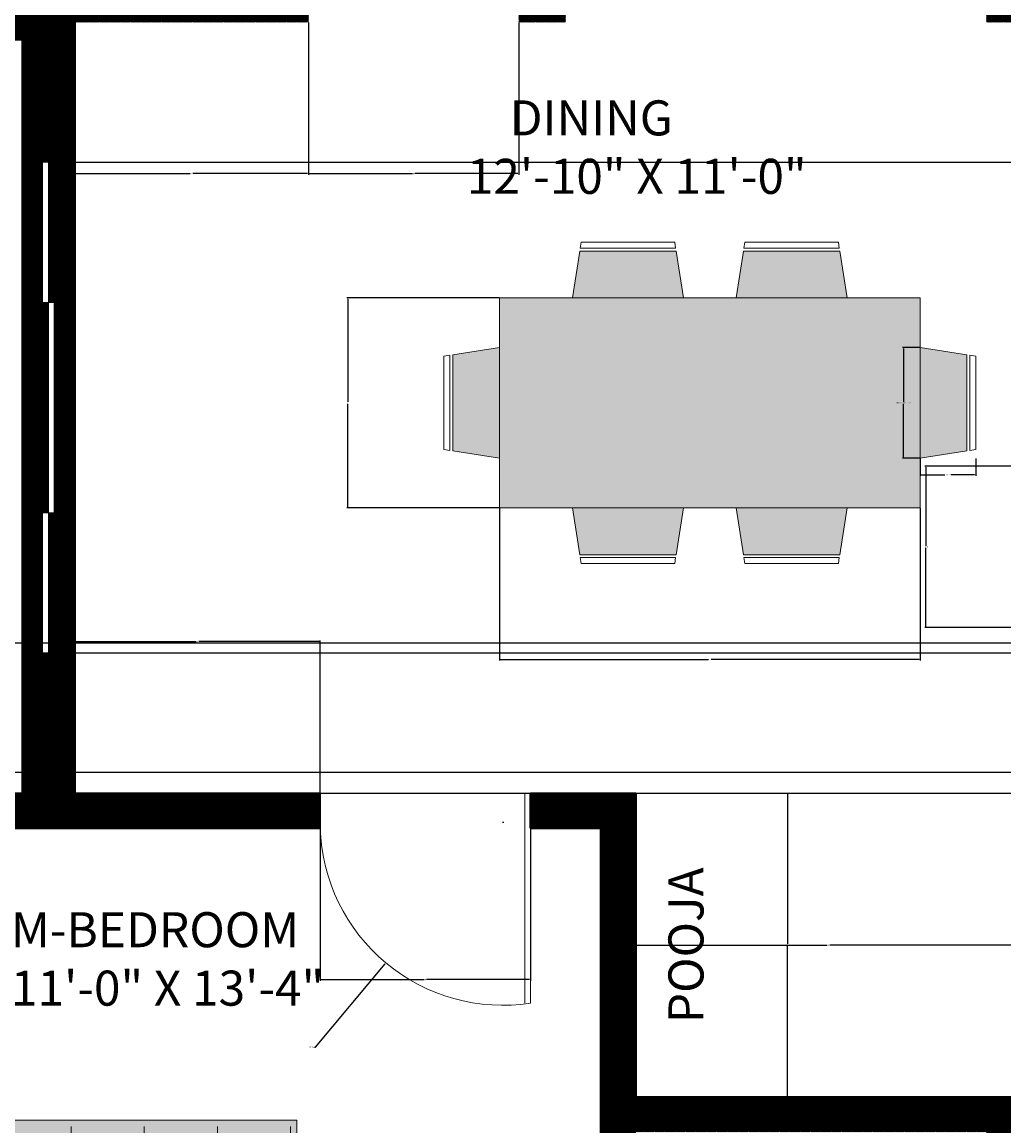
# Model space of a CAD drawing. Units: inches. Extents: x 557 to 1007, y 390 to 953.
# Tile 4 of 10: x 674 to 842, y 558 to 747. Entities that reach past the tile are written whole.
import ezdxf

# ---------------------------------------------------------------- set-up
doc = ezdxf.new("R2010")
doc.units = ezdxf.units.IN
doc.header["$LTSCALE"] = 5
doc.header["$MEASUREMENT"] = 0
for name, color, linetype, lineweight in [('A-ANNO-DIMS', 2, 'Continuous', 18), ('A-AREA-IDEN', 7, 'Continuous', 18), ('A-DOOR', 3, 'Continuous', 18), ('A-FURN', 8, 'Continuous', 18), ('A-FURN-PATT', 9, 'Continuous', 9), ('A-WALL', 7, 'Continuous', 35)]:
    doc.layers.add(name, color=color, linetype=linetype, lineweight=lineweight)
doc.layers.add('A-GLAZ-PATT', color=141, linetype='Continuous', lineweight=9, true_color=0xadddf7)
doc.layers.add('A-WALL-PATT', color=251, linetype='Continuous', lineweight=9, true_color=0x636466)
doc.styles.get("Standard").update_dxf_attribs({"font": 'arial.ttf'})
doc.dimstyles.get("Standard").update_dxf_attribs({"dimtxt": 0.18, "dimasz": 0.18, "dimexe": 0.18, "dimexo": 0.0625, "dimgap": 0.09, "dimtad": 0, "dimtih": 1, "dimtoh": 1, "dimdec": 4, "dimzin": 0, "dimdsep": 46, "dimtxsty": 'Standard', "dimcen": 0.09, "dimadec": 0, "dimazin": 0, "dimtfac": 1, "dimtdec": 4, "dimtofl": 0, "dimtmove": 0, "dimatfit": 3, "dimfxl": 1, "dimtolj": 1, "dimtzin": 0, "dimarcsym": 0})

# ---------------------------------------------------------------- blocks, each defined once
blk = doc.blocks.new('BED-QUEEN-60x80-PLAN')
for p, q in [((0, 0), (0, 60)), ((0, 60), (80, 60)), ((29.6, 60), (14.4, 44.8)), ((29.6, 44.8), (29.6, 60)), ((80, 60), (80, 0)), ((1.2, 52), (16.4, 52)), ((1.2, 31.2), (1.2, 52)), ((16.4, 52), (16.4, 46.8)), ((14.4, 0), (14.4, 44.8)), ((14.4, 44.8), (29.6, 44.8)), ((16.8, 44.8), (16.8, 0)), ((14.4, 31.2), (1.2, 31.2)), ((1.2, 28.8), (14.4, 28.8)), ((1.2, 8), (1.2, 28.8)), ((14.4, 8), (1.2, 8)), ((80, 0), (0, 0))]:
    blk.add_line(p, q)
blk = doc.blocks.new('CHAIR-DINING-PLAN')
for p, q in [((1.48, 9.5), (1.33, 8.5)), ((1.48, 9.5), (17.48, 9.5)), ((17.64, 8.5), (17.48, 9.5)), ((1.25, 8), (0, 0)), ((1.25, 8), (17.72, 8)), ((17.64, 8.5), (1.33, 8.5)), ((18.97, 0), (17.72, 8))]:
    blk.add_line(p, q)
blk = doc.blocks.new('*D25')
at = {"layer": 'A-ANNO-DIMS', "color": 0, "lineweight": -2, "ltscale": 5, "transparency": 16777216}
for p, q in [((828.02, 691.19), (825.05, 691.19)), ((825.23, 691.01), (825.23, 681.89)), ((825.23, 672.41), (825.23, 681.53)), ((828.02, 672.23), (825.05, 672.23))]:
    blk.add_line(p, q, dxfattribs=at)
at = {"layer": 'A-ANNO-DIMS', "color": 0, "ltscale": 5, "transparency": 16777216}
for points in [[(825.2, 691.01), (825.26, 691.01), (825.23, 691.19)], [(825.2, 672.41), (825.26, 672.41), (825.23, 672.23)]]:
    blk.add_solid(points, dxfattribs=at)
at = {"layer": 'Defpoints', "color": 0, "ltscale": 5, "transparency": 16777216}
for p in [(828.08, 691.19), (825.23, 672.23), (828.08, 672.23)]:
    blk.add_point(p, dxfattribs=at)
at = {"layer": 'A-ANNO-DIMS', "color": 0, "ltscale": 5, "transparency": 16777216, "insert": (825.23, 681.71), "char_height": 0.18, "attachment_point": 5}
blk.add_mtext('\\A1;DINING CHAIR 19 TYP.', dxfattribs=at)
blk = doc.blocks.new('*D26')
at = {"layer": 'A-ANNO-DIMS', "color": 0, "lineweight": -2, "ltscale": 5, "transparency": 16777216}
for p, q in [((828.08, 672.16), (828.08, 669.2)), ((837.58, 672.16), (837.58, 669.2)), ((828.26, 669.38), (832.31, 669.38)), ((837.4, 669.38), (833.35, 669.38))]:
    blk.add_line(p, q, dxfattribs=at)
at = {"layer": 'A-ANNO-DIMS', "color": 0, "ltscale": 5, "transparency": 16777216}
for points in [[(828.26, 669.41), (828.26, 669.35), (828.08, 669.38)], [(837.4, 669.41), (837.4, 669.35), (837.58, 669.38)]]:
    blk.add_solid(points, dxfattribs=at)
at = {"layer": 'Defpoints', "color": 0, "ltscale": 5, "transparency": 16777216}
for p in [(828.08, 672.23), (837.58, 672.23), (837.58, 669.38)]:
    blk.add_point(p, dxfattribs=at)
at = {"layer": 'A-ANNO-DIMS', "color": 0, "ltscale": 5, "transparency": 16777216, "insert": (832.83, 669.38), "char_height": 0.18, "attachment_point": 5}
blk.add_mtext('\\A1;10 TYP.', dxfattribs=at)
blk = doc.blocks.new('*D45')
at = {"layer": 'A-ANNO-DIMS', "color": 0, "lineweight": -2, "ltscale": 5, "transparency": 16777216}
for p, q in [((582.82, 605.84), (582.82, 389.77)), ((980.41, 439.84), (980.41, 389.77)), ((583, 389.95), (781.22, 389.95)), ((980.23, 389.95), (782.01, 389.95))]:
    blk.add_line(p, q, dxfattribs=at)
at = {"layer": 'A-ANNO-DIMS', "color": 0, "ltscale": 5, "transparency": 16777216}
for points in [[(583, 389.98), (583, 389.92), (582.82, 389.95)], [(980.23, 389.98), (980.23, 389.92), (980.41, 389.95)]]:
    blk.add_solid(points, dxfattribs=at)
at = {"layer": 'Defpoints', "color": 0, "ltscale": 5, "transparency": 16777216}
for p in [(582.82, 605.9), (980.41, 439.9), (980.41, 389.95)]:
    blk.add_point(p, dxfattribs=at)
at = {"layer": 'A-ANNO-DIMS', "color": 0, "ltscale": 5, "transparency": 16777216, "insert": (781.61, 389.95), "char_height": 0.18, "attachment_point": 5}
blk.add_mtext('\\A1;397.6', dxfattribs=at)
blk = doc.blocks.new('*D46')
at = {"layer": 'A-ANNO-DIMS', "color": 0, "lineweight": -2, "ltscale": 5, "transparency": 16777216}
for p, q in [((761.34, 926.9), (556.69, 926.9)), ((556.87, 926.72), (556.87, 671.59)), ((556.87, 416.08), (556.87, 671.22)), ((773.34, 415.9), (556.69, 415.9))]:
    blk.add_line(p, q, dxfattribs=at)
at = {"layer": 'A-ANNO-DIMS', "color": 0, "ltscale": 5, "transparency": 16777216}
for points in [[(556.84, 926.72), (556.9, 926.72), (556.87, 926.9)], [(556.84, 416.08), (556.9, 416.08), (556.87, 415.9)]]:
    blk.add_solid(points, dxfattribs=at)
at = {"layer": 'Defpoints', "color": 0, "ltscale": 5, "transparency": 16777216}
for p in [(556.87, 926.9), (761.41, 926.9), (773.41, 415.9)]:
    blk.add_point(p, dxfattribs=at)
at = {"layer": 'A-ANNO-DIMS', "color": 0, "ltscale": 5, "transparency": 16777216, "insert": (556.87, 671.4), "char_height": 0.18, "attachment_point": 5}
blk.add_mtext('\\A1;511', dxfattribs=at)
blk = doc.blocks.new('*D60')
at = {"layer": 'A-ANNO-DIMS', "color": 0, "lineweight": -2, "ltscale": 5, "transparency": 16777216}
for p, q in [((683.47, 722.9), (1006.54, 722.9)), ((1006.36, 722.72), (1006.36, 681.09)), ((1006.36, 639.08), (1006.36, 680.72)), ((683.47, 638.9), (1006.54, 638.9))]:
    blk.add_line(p, q, dxfattribs=at)
at = {"layer": 'A-ANNO-DIMS', "color": 0, "ltscale": 5, "transparency": 16777216}
for points in [[(1006.33, 722.72), (1006.39, 722.72), (1006.36, 722.9)], [(1006.33, 639.08), (1006.39, 639.08), (1006.36, 638.9)]]:
    blk.add_solid(points, dxfattribs=at)
at = {"layer": 'Defpoints', "color": 0, "ltscale": 5, "transparency": 16777216}
for p in [(683.41, 722.9), (683.41, 638.9), (1006.36, 638.9)]:
    blk.add_point(p, dxfattribs=at)
at = {"layer": 'A-ANNO-DIMS', "color": 0, "ltscale": 5, "transparency": 16777216, "insert": (1006.36, 680.9), "char_height": 0.18, "attachment_point": 5}
blk.add_mtext('\\A1;84', dxfattribs=at)
blk = doc.blocks.new('*D61')
at = {"layer": 'A-ANNO-DIMS', "color": 0, "lineweight": -2, "ltscale": 5, "transparency": 16777216}
for p, q in [((683.47, 638.9), (1006.54, 638.9)), ((1006.36, 638.72), (1006.36, 627.08)), ((1006.36, 615.08), (1006.36, 626.72)), ((683.47, 614.9), (1006.54, 614.9))]:
    blk.add_line(p, q, dxfattribs=at)
at = {"layer": 'A-ANNO-DIMS', "color": 0, "ltscale": 5, "transparency": 16777216}
for points in [[(1006.33, 638.72), (1006.39, 638.72), (1006.36, 638.9)], [(1006.33, 615.08), (1006.39, 615.08), (1006.36, 614.9)]]:
    blk.add_solid(points, dxfattribs=at)
at = {"layer": 'Defpoints', "color": 0, "ltscale": 5, "transparency": 16777216}
for p in [(683.41, 638.9), (683.41, 614.9), (1006.36, 614.9)]:
    blk.add_point(p, dxfattribs=at)
at = {"layer": 'A-ANNO-DIMS', "color": 0, "ltscale": 5, "transparency": 16777216, "insert": (1006.36, 626.9), "char_height": 0.18, "attachment_point": 5}
blk.add_mtext('\\A1;24', dxfattribs=at)
blk = doc.blocks.new('*D62')
at = {"layer": 'A-ANNO-DIMS', "color": 0, "lineweight": -2, "ltscale": 5, "transparency": 16777216}
for p, q in [((756.08, 663.65), (756.08, 637.58)), ((828.08, 663.65), (828.08, 637.58)), ((756.26, 637.76), (791.86, 637.76)), ((827.9, 637.76), (792.3, 637.76))]:
    blk.add_line(p, q, dxfattribs=at)
at = {"layer": 'A-ANNO-DIMS', "color": 0, "ltscale": 5, "transparency": 16777216}
for points in [[(756.26, 637.79), (756.26, 637.73), (756.08, 637.76)], [(827.9, 637.79), (827.9, 637.73), (828.08, 637.76)]]:
    blk.add_solid(points, dxfattribs=at)
at = {"layer": 'Defpoints', "color": 0, "ltscale": 5, "transparency": 16777216}
for p in [(756.08, 663.71), (828.08, 663.71), (756.08, 637.76)]:
    blk.add_point(p, dxfattribs=at)
at = {"layer": 'A-ANNO-DIMS', "color": 0, "ltscale": 5, "transparency": 16777216, "insert": (792.08, 637.76), "char_height": 0.18, "attachment_point": 5}
blk.add_mtext('\\A1;72', dxfattribs=at)
blk = doc.blocks.new('*D63')
at = {"layer": 'A-ANNO-DIMS', "color": 0, "lineweight": -2, "ltscale": 5, "transparency": 16777216}
for p, q in [((756.02, 699.71), (729.95, 699.71)), ((730.13, 699.53), (730.13, 681.89)), ((730.13, 663.89), (730.13, 681.53)), ((756.02, 663.71), (729.95, 663.71))]:
    blk.add_line(p, q, dxfattribs=at)
at = {"layer": 'A-ANNO-DIMS', "color": 0, "ltscale": 5, "transparency": 16777216}
for points in [[(730.1, 699.53), (730.16, 699.53), (730.13, 699.71)], [(730.1, 663.89), (730.16, 663.89), (730.13, 663.71)]]:
    blk.add_solid(points, dxfattribs=at)
at = {"layer": 'Defpoints', "color": 0, "ltscale": 5, "transparency": 16777216}
for p in [(730.13, 699.71), (756.08, 699.71), (756.08, 663.71)]:
    blk.add_point(p, dxfattribs=at)
at = {"layer": 'A-ANNO-DIMS', "color": 0, "ltscale": 5, "transparency": 16777216, "insert": (730.13, 681.71), "char_height": 0.18, "attachment_point": 5}
blk.add_mtext('\\A1;36', dxfattribs=at)
blk = doc.blocks.new('*D69')
at = {"layer": 'A-ANNO-DIMS', "color": 0, "lineweight": -2, "ltscale": 5, "transparency": 16777216}
for p, q in [((723.41, 746.84), (723.41, 720.77)), ((759.41, 746.84), (759.41, 720.77)), ((723.59, 720.95), (741.19, 720.95)), ((759.23, 720.95), (741.62, 720.95))]:
    blk.add_line(p, q, dxfattribs=at)
at = {"layer": 'A-ANNO-DIMS', "color": 0, "ltscale": 5, "transparency": 16777216}
for points in [[(723.59, 720.98), (723.59, 720.92), (723.41, 720.95)], [(759.23, 720.98), (759.23, 720.92), (759.41, 720.95)]]:
    blk.add_solid(points, dxfattribs=at)
at = {"layer": 'Defpoints', "color": 0, "ltscale": 5, "transparency": 16777216}
for p in [(723.41, 746.9), (759.41, 746.9), (723.41, 720.95)]:
    blk.add_point(p, dxfattribs=at)
at = {"layer": 'A-ANNO-DIMS', "color": 0, "ltscale": 5, "transparency": 16777216, "insert": (741.41, 720.95), "char_height": 0.18, "attachment_point": 5}
blk.add_mtext('\\A1;36', dxfattribs=at)
blk = doc.blocks.new('*D72')
at = {"layer": 'A-ANNO-DIMS', "color": 0, "lineweight": -2, "ltscale": 5, "transparency": 16777216}
for p, q in [((725.41, 608.84), (725.41, 582.77)), ((761.41, 608.84), (761.41, 582.77)), ((725.59, 582.95), (743.19, 582.95)), ((761.23, 582.95), (743.62, 582.95))]:
    blk.add_line(p, q, dxfattribs=at)
at = {"layer": 'A-ANNO-DIMS', "color": 0, "ltscale": 5, "transparency": 16777216}
for points in [[(725.59, 582.98), (725.59, 582.92), (725.41, 582.95)], [(761.23, 582.98), (761.23, 582.92), (761.41, 582.95)]]:
    blk.add_solid(points, dxfattribs=at)
at = {"layer": 'Defpoints', "color": 0, "ltscale": 5, "transparency": 16777216}
for p in [(725.41, 608.9), (761.41, 608.9), (725.41, 582.95)]:
    blk.add_point(p, dxfattribs=at)
at = {"layer": 'A-ANNO-DIMS', "color": 0, "ltscale": 5, "transparency": 16777216, "insert": (743.41, 582.95), "char_height": 0.18, "attachment_point": 5}
blk.add_mtext('\\A1;36', dxfattribs=at)
blk = doc.blocks.new('*D78')
at = {"layer": 'A-ANNO-DIMS', "color": 0, "lineweight": -2, "ltscale": 5, "transparency": 16777216}
for p, q in [((779.41, 562.97), (779.41, 589.03)), ((779.59, 588.85), (812.19, 588.85)), ((845.23, 588.85), (812.62, 588.85)), ((845.41, 562.97), (845.41, 589.03))]:
    blk.add_line(p, q, dxfattribs=at)
at = {"layer": 'A-ANNO-DIMS', "color": 0, "ltscale": 5, "transparency": 16777216}
for points in [[(779.59, 588.88), (779.59, 588.82), (779.41, 588.85)], [(845.23, 588.88), (845.23, 588.82), (845.41, 588.85)]]:
    blk.add_solid(points, dxfattribs=at)
at = {"layer": 'Defpoints', "color": 0, "ltscale": 5, "transparency": 16777216}
for p in [(845.41, 588.85), (779.41, 562.9), (845.41, 562.9)]:
    blk.add_point(p, dxfattribs=at)
at = {"layer": 'A-ANNO-DIMS', "color": 0, "ltscale": 5, "transparency": 16777216, "insert": (812.41, 588.85), "char_height": 0.18, "attachment_point": 5}
blk.add_mtext('\\A1;66', dxfattribs=at)
blk = doc.blocks.new('*D79')
at = {"layer": 'A-ANNO-DIMS', "color": 0, "lineweight": -2, "ltscale": 5, "transparency": 16777216}
for p, q in [((779.47, 614.9), (805.54, 614.9)), ((805.36, 614.72), (805.36, 589.09)), ((805.36, 563.08), (805.36, 588.72)), ((779.47, 562.9), (805.54, 562.9))]:
    blk.add_line(p, q, dxfattribs=at)
at = {"layer": 'A-ANNO-DIMS', "color": 0, "ltscale": 5, "transparency": 16777216}
for points in [[(805.33, 614.72), (805.39, 614.72), (805.36, 614.9)], [(805.33, 563.08), (805.39, 563.08), (805.36, 562.9)]]:
    blk.add_solid(points, dxfattribs=at)
at = {"layer": 'Defpoints', "color": 0, "ltscale": 5, "transparency": 16777216}
for p in [(779.41, 614.9), (779.41, 562.9), (805.36, 562.9)]:
    blk.add_point(p, dxfattribs=at)
at = {"layer": 'A-ANNO-DIMS', "color": 0, "ltscale": 5, "transparency": 16777216, "insert": (805.36, 588.9), "char_height": 0.18, "attachment_point": 5}
blk.add_mtext('\\A1;52', dxfattribs=at)
blk = doc.blocks.new('*D81')
at = {"layer": 'A-ANNO-DIMS', "color": 0, "lineweight": -2, "ltscale": 5, "transparency": 16777216}
for p, q in [((874.87, 640.54), (556.69, 640.54)), ((556.87, 640.36), (556.87, 629.66)), ((556.87, 618.59), (556.87, 629.29)), ((870.87, 618.41), (556.69, 618.41))]:
    blk.add_line(p, q, dxfattribs=at)
at = {"layer": 'A-ANNO-DIMS', "color": 0, "ltscale": 5, "transparency": 16777216}
for points in [[(556.84, 640.36), (556.9, 640.36), (556.87, 640.54)], [(556.84, 618.59), (556.9, 618.59), (556.87, 618.41)]]:
    blk.add_solid(points, dxfattribs=at)
at = {"layer": 'Defpoints', "color": 0, "ltscale": 5, "transparency": 16777216}
for p in [(874.93, 640.54), (556.87, 618.41), (870.93, 618.41)]:
    blk.add_point(p, dxfattribs=at)
at = {"layer": 'A-ANNO-DIMS', "color": 0, "ltscale": 5, "transparency": 16777216, "insert": (556.87, 629.48), "char_height": 0.18, "attachment_point": 5}
blk.add_mtext('\\A1;22.13', dxfattribs=at)
blk = doc.blocks.new('*D83')
at = {"layer": 'A-ANNO-DIMS', "color": 0, "lineweight": -2, "ltscale": 5, "transparency": 16777216}
for p, q in [((854.95, 670.88), (828.88, 670.88)), ((829.06, 670.7), (829.06, 657.24)), ((829.06, 643.42), (829.06, 656.88)), ((854.95, 643.24), (828.88, 643.24))]:
    blk.add_line(p, q, dxfattribs=at)
at = {"layer": 'A-ANNO-DIMS', "color": 0, "ltscale": 5, "transparency": 16777216}
for points in [[(829.03, 670.7), (829.09, 670.7), (829.06, 670.88)], [(829.03, 643.42), (829.09, 643.42), (829.06, 643.24)]]:
    blk.add_solid(points, dxfattribs=at)
at = {"layer": 'Defpoints', "color": 0, "ltscale": 5, "transparency": 16777216}
for p in [(829.06, 670.88), (855.01, 670.88), (855.01, 643.24)]:
    blk.add_point(p, dxfattribs=at)
at = {"layer": 'A-ANNO-DIMS', "color": 0, "ltscale": 5, "transparency": 16777216, "insert": (829.06, 657.06), "char_height": 0.18, "attachment_point": 5}
blk.add_mtext('\\A1;27.634', dxfattribs=at)
blk = doc.blocks.new('*D98')
at = {"layer": 'A-ANNO-DIMS', "color": 0, "lineweight": -2, "ltscale": 5, "transparency": 16777216}
for p, q in [((683.41, 746.84), (683.41, 720.77)), ((723.41, 746.84), (723.41, 720.77)), ((683.59, 720.95), (703.18, 720.95)), ((723.23, 720.95), (703.63, 720.95))]:
    blk.add_line(p, q, dxfattribs=at)
at = {"layer": 'A-ANNO-DIMS', "color": 0, "ltscale": 5, "transparency": 16777216}
for points in [[(683.59, 720.98), (683.59, 720.92), (683.41, 720.95)], [(723.23, 720.98), (723.23, 720.92), (723.41, 720.95)]]:
    blk.add_solid(points, dxfattribs=at)
at = {"layer": 'Defpoints', "color": 0, "ltscale": 5, "transparency": 16777216}
for p in [(683.41, 746.9), (723.41, 746.9), (683.41, 720.95)]:
    blk.add_point(p, dxfattribs=at)
at = {"layer": 'A-ANNO-DIMS', "color": 0, "ltscale": 5, "transparency": 16777216, "insert": (703.41, 720.95), "char_height": 0.18, "attachment_point": 5}
blk.add_mtext('\\A1;40', dxfattribs=at)
blk = doc.blocks.new('*D100')
at = {"layer": 'A-ANNO-DIMS', "color": 0, "lineweight": -2, "ltscale": 5, "transparency": 16777216}
for p, q in [((683.41, 614.97), (683.41, 641.03)), ((683.59, 640.85), (704.18, 640.85)), ((725.23, 640.85), (704.63, 640.85)), ((725.41, 614.97), (725.41, 641.03))]:
    blk.add_line(p, q, dxfattribs=at)
at = {"layer": 'A-ANNO-DIMS', "color": 0, "ltscale": 5, "transparency": 16777216}
for points in [[(683.59, 640.88), (683.59, 640.82), (683.41, 640.85)], [(725.23, 640.88), (725.23, 640.82), (725.41, 640.85)]]:
    blk.add_solid(points, dxfattribs=at)
at = {"layer": 'Defpoints', "color": 0, "ltscale": 5, "transparency": 16777216}
for p in [(725.41, 640.85), (683.41, 614.9), (725.41, 614.9)]:
    blk.add_point(p, dxfattribs=at)
at = {"layer": 'A-ANNO-DIMS', "color": 0, "ltscale": 5, "transparency": 16777216, "insert": (704.41, 640.85), "char_height": 0.18, "attachment_point": 5}
blk.add_mtext('\\A1;42', dxfattribs=at)
blk = doc.blocks.new('*D109')
at = {"layer": 'A-ANNO-DIMS', "color": 0, "lineweight": -2, "ltscale": 5, "transparency": 16777216}
for p, q in [((756.63, 609.89), (756.81, 609.89)), ((756.72, 609.8), (756.72, 609.98)), ((724.63, 571.37), (736.55, 585.68)), ((724.45, 571.37), (724.63, 571.37))]:
    blk.add_line(p, q, dxfattribs=at)
at = {"layer": 'A-ANNO-DIMS', "color": 0, "ltscale": 5, "transparency": 16777216}
blk.add_solid([(736.53, 585.7), (736.57, 585.66), (736.66, 585.82)], dxfattribs=at)
at = {"layer": 'Defpoints', "color": 0, "ltscale": 5, "transparency": 16777216}
for p in [(756.72, 609.89), (736.66, 585.82)]:
    blk.add_point(p, dxfattribs=at)
at = {"layer": 'A-ANNO-DIMS', "color": 0, "ltscale": 5, "transparency": 16777216, "insert": (723.9, 571.37), "char_height": 0.18, "attachment_point": 5}
blk.add_mtext('\\A1;R31.334', dxfattribs=at)

msp = doc.modelspace()

# ---------------------------------------------------------------- hatches: boundary and pattern name
at = {"layer": 'A-FURN-PATT', "ltscale": 5}
h = msp.add_hatch(dxfattribs=at)
h.set_pattern_fill('GRAVEL', color=256, scale=25)
h.set_pattern_definition([(228.01279, (18, 25), (-200, -225), [3.3634, -332.9772]), (184.96974, (15.75, 22.5), (300, 25), [5.7717, -571.39812]), (132.51045, (10, 22), (250, -275), [4.0697, -402.9008]), (267.27369, (0.25, 15.75), (25, 500), [5.25595, -520.33895]), (292.83365, (0, 10.5), (-125, 300), [5.15387, -510.23433]), (357.27369, (2, 5.75), (-500, 25), [5.25595, -520.33895]), (37.69424, (7.25, 5.5), (-325, -250), [6.95072, -688.1212]), (72.25533, (12.75, 9.75), (175, 550), [6.5622, -649.65804]), (121.42957, (14.75, 16), (-200, 325), [5.27375, -522.10183]), (175.23636, (12, 20.5), (275, -25), [6.0208, -295.01906]), (222.39744, (6, 21), (-300, -275), [7.7862, -770.83438]), (138.81407, (25, 15.5), (-175, 150), [2.65752, -263.0961]), (171.46923, (23, 17.25), (325, -50), [5.05593, -500.5378]), (225, (18, 18), (-3e-15, -25), [3.53552, -31.8198]), (203.1986, (16.25, 21), (125, 50), [1.90395, -188.49038]), (291.8014, (14.5, 20.25), (-25, 75), [2.69257, -131.93655]), (30.96376, (15.5, 17.75), (75, 50), [4.37322, -141.40057]), (161.56505, (19.25, 20), (50, -25), [3.16228, -75.89467]), (16.38954, (0, 20.25), (250, 75), [4.43, -438.57113]), (70.34618, (4.25, 21.5), (-100, -275), [3.71652, -367.9352]), (293.1986, (19.25, 25), (-50, 125), [3.80788, -186.58645]), (343.61046, (20.75, 21.5), (-250, 75), [4.43, -438.57113]), (339.44395, (0, 4.75), (-125, 50), [4.272, -209.3281]), (294.77514, (4, 3.25), (-125, 275), [3.57945, -354.36608]), (66.8014, (19.5, 0), (50, 125), [3.80788, -186.58645]), (17.35402, (21, 3.5), (-325, -100), [4.19078, -414.8856]), (69.44395, (7.25, 0), (-50, -125), [2.136, -211.4641]), (101.30993, (18, 0), (-25, 100), [1.27475, -126.20074]), (165.96376, (17.75, 1.25), (75, -25), [5.15388, -97.92377]), (186.00901, (12.75, 2.5), (250, 25), [4.77625, -472.84808]), (303.69007, (15.5, 15.5), (-25, 50), [3.60555, -86.53323]), (353.15723, (17.5, 12.5), (425, -50), [6.29485, -623.18907]), (60.9454, (23.75, 11.75), (-100, -175), [2.5739, -254.81685]), (90, (25, 14), (-25, 25), [1.5, -23.5]), (120.25644, (12.25, 3.25), (100, -175), [3.4731, -343.838]), (48.01279, (10.5, 6.25), (200, 225), [6.7268, -329.6138]), (0, (15, 11.25), (25, 25), [6.5, -18.5]), (325.30485, (21.5, 11.25), (250, -175), [3.95285, -391.33186]), (254.0546, (24.75, 9), (-25, -100), [3.64005, -178.3627]), (207.64598, (23.75, 5.5), (-475, -250), [5.92662, -586.73685]), (175.42608, (18.5, 2.75), (-325, 25), [6.26997, -620.72684])])
h.paths.add_polyline_path([(615.2525, 688.5, 1), (640.7475, 688.5, 1)])
h.paths.add_polyline_path([(917.0544, 663.8414, 0.33333323), (915.2241, 665.6717), (882.2793, 665.6717, 0.33333323), (880.449, 663.8414), (880.449, 649.1992, 0.33333323), (882.2793, 647.369), (915.2241, 647.369, 0.33333323), (917.0544, 649.1992)])
h.paths.add_polyline_path([(828.0807, 699.7098), (756.0807, 699.7098), (756.0807, 663.7098), (828.0807, 663.7098)])
h.paths.add_polyline_path([(787.5651, 663.7098), (768.5964, 663.7098), (769.8463, 655.7098), (786.3151, 655.7098)])
h.paths.add_polyline_path([(815.5651, 663.7098), (796.5964, 663.7098), (797.8463, 655.7098), (814.3151, 655.7098)])
h.paths.add_polyline_path([(836.0807, 689.9442), (828.0807, 691.1942), (828.0807, 672.2255), (836.0807, 673.4755)])
h.paths.add_polyline_path([(756.0807, 691.1942), (748.0807, 689.9442), (748.0807, 673.4755), (756.0807, 672.2255)])
h.paths.add_polyline_path([(786.3151, 707.7098), (769.8463, 707.7098), (768.5964, 699.7098), (787.5651, 699.7098)])
h.paths.add_polyline_path([(814.3151, 707.7098), (797.8463, 707.7098), (796.5964, 699.7098), (815.5651, 699.7098)])
h.paths.add_polyline_path([(917.4362, 607.3575), (889.5896, 607.3575), (889.5896, 586.4726), (917.4362, 586.4726)])
h.paths.add_polyline_path([(721.4053, 881.8539), (671.0053, 881.8539), (671.0053, 866.6539), (658.2053, 866.6539), (658.2053, 821.8539), (721.4053, 821.8539)])
h.paths.add_polyline_path([(925.4053, 875.1046), (875.0053, 875.1046), (875.0053, 859.9046), (862.2053, 859.9046), (862.2053, 815.1046), (925.4053, 815.1046)])
h.paths.add_polyline_path([(721.4053, 558.9046), (671.0053, 558.9046), (671.0053, 543.7046), (658.2053, 543.7046), (658.2053, 498.9046), (721.4053, 498.9046)])
at = {"layer": 'A-FURN-PATT'}
h = msp.add_hatch(dxfattribs=at)
h.set_pattern_fill('CROSS', color=256, scale=25)
h.paths.add_polyline_path([(925.4053, 875.1046), (875.0053, 875.1046), (875.0053, 859.9046), (862.2053, 859.9046), (862.2053, 815.1046), (925.4053, 815.1046)])
h.paths.add_polyline_path([(721.4053, 881.8539), (671.0053, 881.8539), (671.0053, 866.6539), (658.2053, 866.6539), (658.2053, 821.8539), (721.4053, 821.8539)])
h.paths.add_polyline_path([(671.0053, 881.8539), (655.8053, 866.6539), (671.0053, 866.6539)], flags=17)
h.paths.add_polyline_path([(671.0053, 881.8539), (641.4053, 881.8539), (641.4053, 821.8539), (655.8053, 821.8539), (655.8053, 829.8539), (642.6053, 829.8539), (642.6053, 850.6539), (655.8053, 850.6539), (655.8053, 853.0539), (642.6053, 853.0539), (642.6053, 873.8539), (657.8053, 873.8539), (657.8053, 868.6539)])
h.paths.add_polyline_path([(875.0053, 875.1046), (859.8053, 859.9046), (875.0053, 859.9046)], flags=17)
h.paths.add_polyline_path([(875.0053, 875.1046), (845.4053, 875.1046), (845.4053, 815.1046), (859.8053, 815.1046), (859.8053, 823.1046), (846.6053, 823.1046), (846.6053, 843.9046), (859.8053, 843.9046), (859.8053, 846.3046), (846.6053, 846.3046), (846.6053, 867.1046), (861.8053, 867.1046), (861.8053, 861.9046)])
h.paths.add_polyline_path([(721.4053, 558.9046), (671.0053, 558.9046), (671.0053, 543.7046), (658.2053, 543.7046), (658.2053, 498.9046), (721.4053, 498.9046)])
h.paths.add_polyline_path([(671.0053, 558.9046), (641.4053, 558.9046), (641.4053, 498.9046), (655.8053, 498.9046), (655.8053, 506.9046), (642.6053, 506.9046), (642.6053, 527.7046), (655.8053, 527.7046), (655.8053, 530.1046), (642.6053, 530.1046), (642.6053, 550.9046), (657.8053, 550.9046), (657.8053, 545.7046)])
h.paths.add_polyline_path([(671.0053, 558.9046), (657.8053, 545.7046), (655.8053, 543.7046), (671.0053, 543.7046)], flags=17)
h.paths.add_polyline_path([(873.1461, 661.8773, 0.41421356), (868.1461, 666.8773, -0.12244426), (867.1516, 666.8773), (855.014, 666.8773), (855.014, 647.2429), (867.4581, 647.2429, -0.08537395), (868.1461, 647.2429, 0.41421356), (873.1461, 652.2429)])
h.paths.add_polyline_path([(917.0544, 663.8414, 0.33333323), (915.2241, 665.6717), (882.2793, 665.6717, 0.33333323), (880.449, 663.8414), (880.449, 649.1992, 0.33333323), (882.2793, 647.369), (915.2241, 647.369, 0.33333323), (917.0544, 649.1992)])
h.paths.add_polyline_path([(944.9465, 667.5202), (932.6561, 667.5202, -0.10407786), (931.8144, 667.5202, 0.41421356), (926.8144, 662.5202), (926.8144, 652.8858, 0.41421356), (931.8144, 647.8858, -0.05611627), (932.2647, 647.8858), (944.9465, 647.8858)])
h.paths.add_polyline_path([(928.8341, 635.542, 0.41421356), (923.8341, 640.542), (914.1997, 640.542, 0.41421356), (909.1997, 635.542), (909.1997, 622.4099), (923.8341, 622.4099, 0.41421356), (928.8341, 627.4099)])
h.paths.add_polyline_path([(909.1997, 635.542, 0.41421356), (904.1997, 640.542), (894.5653, 640.542, 0.41421356), (889.5653, 635.542), (889.5653, 622.4099), (909.1997, 622.4099)])
h.paths.add_polyline_path([(889.5653, 635.542, 0.41421356), (884.5653, 640.542), (874.9308, 640.542, 0.41421356), (869.9308, 635.542), (869.9308, 627.4099, 0.41421356), (874.9308, 622.4099), (889.5653, 622.4099)])
h = msp.add_hatch(dxfattribs=at)
h.set_pattern_fill('CORK', color=256, scale=25)
h.set_pattern_definition([(0, (0, 0), (0, 3.125), []), (135, (1.5625, -1.5625), (-6.25, -6.25), [4.41942, -4.41942]), (135, (2.344, -1.5625), (-6.25, -6.25), [4.41942, -4.41942]), (135, (3.125, -1.5625), (-6.25, -6.25), [4.41942, -4.41942])])
h.paths.add_polyline_path([(932.8341, 623.4099), (932.8341, 630.9869, 0.76666915), (928.8341, 630.9869), (928.8341, 627.4099), (928.8341, 622.4099), (909.1997, 622.4099), (874.9308, 622.4099), (869.9308, 622.4099), (869.9308, 632.3614, 0.60407544), (865.9308, 632.3614), (865.9308, 623.4099, 0.41421356), (870.9308, 618.4099), (927.8341, 618.4099, 0.41421356)])
h.paths.add_polyline_path([(855.014, 666.8773), (868.1461, 666.8773, 0.78182568), (868.1461, 670.8773), (855.014, 670.8773, 0.41421356), (850.014, 665.8773), (850.014, 648.2429, 0.41421356), (855.014, 643.2429), (868.1461, 643.2429, 0.84268288), (868.1461, 647.2429), (855.014, 647.2429)])
h.paths.add_polyline_path([(948.9465, 666.5202, 0.41421356), (943.9465, 671.5202), (931.8144, 671.5202, 0.81146646), (931.8144, 667.5202), (944.9465, 667.5202), (944.9465, 647.8858), (931.8144, 647.8858, 0.89373088), (931.8144, 643.8858), (943.9465, 643.8858, 0.41421356), (948.9465, 648.8858)])
h.paths.add_polyline_path([(951.6399, 638.9424), (935.2317, 638.9424), (935.2317, 622.9231), (951.6399, 622.9231)])
h.paths.add_polyline_path([(947.0475, 626.5028), (947.0441, 626.4915), (947.0523, 626.4868)], flags=16)
h.paths.add_polyline_path([(944.6349, 630.5579), (944.0837, 633.55), (944.1177, 633.5282), (944.0932, 633.4983), (944.6349, 630.5579), (947.5056, 631.5148), (947.5212, 631.5348), (947.5189, 631.5192), (944.6349, 630.5579), (944.8619, 630.2742), (944.9055, 630.2607), (944.8981, 630.2289)], flags=16)
h.paths.add_polyline_path([(863.4458, 638.9424), (847.0376, 638.9424), (847.0376, 622.9231), (863.4458, 622.9231)])
h.paths.add_polyline_path([(858.2228, 627.4003), (858.2193, 627.3889), (858.2276, 627.3842)], flags=16)
h.paths.add_polyline_path([(855.8101, 631.4553), (855.259, 634.4474), (855.2929, 634.4257), (855.2685, 634.3958), (855.8101, 631.4553), (858.6808, 632.4122), (858.6964, 632.4323), (858.6941, 632.4166), (855.8101, 631.4553), (856.0371, 631.1716), (856.0807, 631.1581), (856.0733, 631.1263)], flags=16)
h.paths.add_polyline_path([(638.0774, 656.4227, 0.37705983), (643.354, 656.1836), (656.3799, 666.6283, 0.31001778), (657.6899, 670.9599, 1.23353517)], flags=17)
h.paths.add_polyline_path([(659.8169, 665.539, 0.41421356), (660.4353, 671.1619), (653.5962, 679.6912), (652.0359, 678.44), (654.9689, 674.7822, -0.09486374), (657.6899, 670.9599, -0.31001778), (656.3799, 666.6283), (643.354, 656.1836, -0.37705983), (638.0774, 656.4227, -0.08126294), (635.5314, 659.5452), (632.7686, 662.9907), (631.2083, 661.7396), (638.0474, 653.2104, 0.41421356), (643.6703, 652.592)])
h.paths.add_polyline_path([(646.6056, 722.6678, 0.39517975), (641.1529, 722.2481), (635.2941, 715.8481, 0.75247437), (655.9256, 699.5214), (660.8023, 706.4923, 0.05595903), (661.2292, 707.2762, 0.02810216), (661.5248, 708.7853, 0.22754294), (660.027, 711.9059)])
h.paths.add_polyline_path([(647.072, 726.1392, 0.39517975), (641.6193, 725.7194), (633.4395, 716.7841), (634.9147, 715.4336), (641.1529, 722.2481, -0.39517975), (646.6056, 722.6678), (660.027, 711.9059, -0.22754294), (661.5248, 708.7853, -0.02810216), (661.2292, 707.2762, -0.05595903), (660.8023, 706.4923), (655.9256, 699.5214), (655.5065, 698.9223), (657.1453, 697.7758), (664.0894, 707.702, 0.39517975), (663.3141, 713.1156)])
h.paths.add_polyline_path([(640.7475, 688.5, 1), (615.2525, 688.5, 1)])
at = {"layer": 'A-GLAZ-PATT'}
h = msp.add_hatch(dxfattribs=at)
h.set_pattern_fill('ANSI31', color=256)
h.paths.add_polyline_path([(635.9053, 814.7688), (636.9053, 814.7688), (636.9053, 838.7688), (632.4053, 838.7688), (632.4053, 790.7688), (635.9053, 790.7688)])
h.paths.add_polyline_path([(641.4053, 838.7688), (637.9053, 838.7688), (637.9053, 814.7688), (636.9053, 814.7688), (636.9053, 790.7688), (641.4053, 790.7688)])
h.paths.add_polyline_path([(603.4053, 728.9046, -0.41421356), (623.4053, 748.9046), (632.4053, 748.9046), (632.4053, 752.9046), (623.4053, 752.9046, 0.41421356), (599.4053, 728.9046), (599.4053, 614.9046), (603.4053, 614.9046)])
h.paths.add_polyline_path([(632.4053, 743.9046), (632.4053, 747.9046), (623.4053, 747.9046, 0.41421356), (604.4053, 728.9046), (604.4053, 614.9046), (608.4053, 614.9046), (608.4053, 719.9046, -0.41421356)])
h.paths.add_polyline_path([(683.4053, 722.9046), (678.9053, 722.9046), (678.9053, 698.9046), (679.9053, 698.9046), (679.9053, 662.9046), (678.9053, 662.9046), (678.9053, 638.9046), (683.4053, 638.9046)])
h.paths.add_polyline_path([(678.9053, 698.9046), (677.9053, 698.9046), (677.9053, 722.9046), (674.4053, 722.9046), (674.4053, 638.9046), (677.9053, 638.9046), (677.9053, 662.9046), (678.9053, 662.9046)])
h.paths.add_polyline_path([(635.9053, 593.9046), (632.4053, 593.9046), (632.4053, 557.9046), (635.9053, 557.9046)])
h.paths.add_polyline_path([(641.4053, 593.9046), (637.9053, 593.9046), (637.9053, 557.9046), (641.4053, 557.9046)])
h.paths.add_polyline_path([(764.9579, 448.9046), (716.9579, 448.9046), (716.9579, 445.4046), (740.9579, 445.4046), (740.9579, 444.4046), (764.9579, 444.4046)])
h.paths.add_polyline_path([(764.9579, 443.4046), (740.9579, 443.4046), (740.9579, 444.4046), (716.9579, 444.4046), (716.9579, 439.9046), (764.9579, 439.9046)])
h.paths.add_polyline_path([(938.4053, 905.9046), (878.4053, 905.9046), (878.4053, 902.4046), (908.4053, 902.4046), (908.4053, 901.4046), (938.4053, 901.4046)])
h.paths.add_polyline_path([(938.4053, 900.4046), (908.4053, 900.4046), (908.4053, 901.4046), (878.4053, 901.4046), (878.4053, 896.9046), (938.4053, 896.9046)])
h.paths.add_polyline_path([(724.9087, 905.9046), (676.9087, 905.9046), (676.9087, 902.4046), (701.4053, 902.4046), (701.4053, 901.4046), (724.9087, 901.4046)])
h.paths.add_polyline_path([(724.9087, 900.4046), (701.4053, 900.4046), (701.4053, 901.4046), (676.9087, 901.4046), (676.9087, 896.9046), (724.9087, 896.9046)])
h.paths.add_polyline_path([(832.0625, 905.9046), (808.0625, 905.9046), (808.0625, 902.4046), (832.0625, 902.4046)])
h.paths.add_polyline_path([(832.0625, 900.4046), (808.0625, 900.4046), (808.0625, 896.9046), (832.0625, 896.9046)])
at = {"layer": 'A-WALL-PATT'}
h = msp.add_hatch(dxfattribs=at)
h.set_pattern_fill('ANSI31', color=256)
h.paths.add_polyline_path([(808.0625, 905.9046), (767.4053, 905.9046), (767.4053, 920.9046), (839.4053, 920.9046), (839.4053, 905.9046), (832.0625, 905.9046), (832.0625, 896.9046), (839.4053, 896.9046), (839.4053, 800.9046), (837.4053, 800.9046), (837.4053, 794.9046), (839.4053, 794.9046), (839.4053, 790.9046), (845.4053, 790.9046), (845.4053, 896.9046), (878.4053, 896.9046), (878.4053, 905.9046), (845.4053, 905.9046), (845.4053, 926.9046), (761.4053, 926.9046), (761.4053, 914.9046), (761.4053, 905.9046), (724.9087, 905.9046), (724.9087, 896.9046), (761.4053, 896.9046), (761.4053, 752.9046), (759.4053, 752.9046), (759.4053, 746.9046), (767.4053, 746.9046), (767.4053, 794.9046), (807.4053, 794.9046), (807.4053, 800.9046), (767.4053, 800.9046), (767.4053, 896.9046), (808.0625, 896.9046)])
h.paths.add_polyline_path([(676.9087, 905.9046), (632.4053, 905.9046), (632.4053, 838.7688), (641.4053, 838.7688), (641.4053, 881.8539), (641.4053, 896.9046), (676.9087, 896.9046)])
h.paths.add_polyline_path([(980.4053, 905.9046), (938.4053, 905.9046), (938.4053, 896.9046), (971.4053, 896.9046), (971.4053, 752.9046), (845.4053, 752.9046), (845.4053, 754.9046), (839.4053, 754.9046), (839.4053, 746.9046), (971.4053, 746.9046), (971.4053, 720.1788), (980.4053, 720.1788)])
h.paths.add_polyline_path([(723.4053, 752.9046), (641.4053, 752.9046), (641.4053, 790.7688), (632.4053, 790.7688), (632.4053, 743.9046), (674.4053, 743.9046), (674.4053, 722.9046), (683.4053, 722.9046), (683.4053, 746.9046), (723.4053, 746.9046)])
h.paths.add_polyline_path([(980.4053, 684.1788), (971.4053, 684.1788), (971.4053, 614.9046), (845.4053, 614.9046), (845.4053, 608.9046), (971.4053, 608.9046), (971.4053, 512.9046), (908.7697, 512.9046), (908.7697, 508.9046), (971.4053, 508.9046), (971.4053, 448.9046), (845.4053, 448.9046), (845.4053, 508.9046), (878.7697, 508.9046), (878.7697, 512.9046), (845.4053, 512.9046), (845.4053, 562.9046), (779.4053, 562.9046), (779.4053, 614.9046), (761.4053, 614.9046), (761.4053, 608.9046), (773.4053, 608.9046), (773.4053, 512.636), (779.4053, 512.636), (779.4053, 556.9046), (839.4053, 556.9046), (839.4053, 448.9046), (830.432, 448.9046), (830.432, 439.9046), (839.4053, 439.9046), (839.4053, 433.0506), (839.4053, 421.9046), (779.4053, 421.9046), (779.4053, 439.9046), (796.9656, 439.9046), (806.432, 439.9046), (806.432, 448.9046), (779.4053, 448.9046), (779.4053, 482.636), (773.4053, 482.636), (773.4053, 448.9046), (764.9579, 448.9046), (764.9579, 439.9046), (773.4053, 439.9046), (773.4053, 415.9046), (845.4053, 415.9046), (845.4053, 439.9046), (980.4053, 439.9046)])
h.paths.add_polyline_path([(716.9579, 448.9046), (641.4053, 448.9046), (641.4053, 557.9046), (632.4053, 557.9046), (632.4053, 439.9046), (716.9579, 439.9046)])
h.paths.add_polyline_path([(725.4053, 614.9046), (683.4053, 614.9046), (683.4053, 638.9046), (674.4053, 638.9046), (674.4053, 614.9046), (608.4053, 614.9046), (582.8236, 614.9046), (582.8236, 605.9046), (599.4053, 605.9046), (632.4053, 605.9046), (641.4053, 605.9046), (641.4053, 608.9046), (725.4053, 608.9046)])
h.paths.add_polyline_path([(641.4053, 605.9046), (632.4053, 605.9046), (632.4053, 593.9046), (641.4053, 593.9046)])

# ---------------------------------------------------------------- linework, layer by layer
at = {"layer": 'A-DOOR'}
for p, q in [((683.4053, 722.9046), (674.4053, 722.9046)), ((677.9053, 722.9046), (677.9053, 698.9046)), ((678.9053, 722.9046), (678.9053, 638.9046)), ((679.9053, 698.9046), (677.9053, 698.9046)), ((679.9053, 698.9046), (679.9053, 662.9046)), ((679.9053, 662.9046), (677.9053, 662.9046)), ((677.9053, 662.9046), (677.9053, 638.9046)), ((683.4053, 638.9046), (674.4053, 638.9046)), ((760.4053, 614.9046), (760.4053, 578.9046)), ((761.4053, 614.9046), (761.4053, 578.9046))]:
    msp.add_line(p, q, dxfattribs=at)
msp.add_arc((756.7242, 609.8873), 31.3344, 181.797233, 278.591625, dxfattribs=at)
at = {"layer": 'A-FURN'}
for p, q in [((828.0807, 699.7098), (756.0807, 699.7098)), ((756.0807, 699.7098), (756.0807, 663.7098)), ((828.0807, 663.7098), (828.0807, 699.7098)), ((756.0807, 663.7098), (828.0807, 663.7098))]:
    msp.add_line(p, q, dxfattribs=at)
at = {"layer": 'A-WALL'}
for p, q in [((683.4053, 746.9046), (683.4053, 614.9046)), ((632.4053, 743.9046), (674.4053, 743.9046)), ((674.4053, 743.9046), (674.4053, 614.9046)), ((608.4053, 614.9046), (674.4053, 614.9046)), ((683.4053, 614.9046), (725.4053, 614.9046)), ((725.4053, 608.9046), (725.4053, 614.9046)), ((761.4053, 608.9046), (761.4053, 614.9046)), ((761.4053, 614.9046), (779.4053, 614.9046)), ((779.4053, 614.9046), (779.4053, 562.9046)), ((641.4053, 608.9046), (725.4053, 608.9046)), ((761.4053, 608.9046), (773.4053, 608.9046)), ((773.4053, 608.9046), (773.4053, 512.636)), ((779.4053, 562.9046), (869.4053, 562.9046))]:
    msp.add_line(p, q, dxfattribs=at)

# ---------------------------------------------------------------- block references
at = {"layer": 'A-FURN'}
for name, p in [('CHAIR-DINING-PLAN', (768.596, 699.707)), ('CHAIR-DINING-PLAN', (796.596, 699.707)), ('BED-QUEEN-60x80-PLAN', (641.405, 498.905))]:
    msp.add_blockref(name, p, dxfattribs=at)
at = {"layer": 'A-FURN', "extrusion": (0, 0, -1), "zscale": -1}
for p, rotation in [((-756.0835, 691.1945), 270.0000035370376), ((-768.596, 663.7127), 180), ((-796.596, 663.7127), 180)]:
    msp.add_blockref('CHAIR-DINING-PLAN', p, dxfattribs=dict(at, rotation=rotation))
at = {"layer": 'A-FURN', "rotation": 269.9999613072867}
msp.add_blockref('CHAIR-DINING-PLAN', (828.0779, 691.1946), dxfattribs=at)

# ---------------------------------------------------------------- texts
at = {"layer": 'A-AREA-IDEN', "char_height": 6, "attachment_point": 1}
for s, insert in [('    DINING\\P12\'-10" X 11\'-0"', (750.5, 733.5)), ('M-BEDROOM\\P11\'-0" X 13\'-4"', (672.5, 594.5))]:
    msp.add_mtext_dynamic_manual_height_columns(s, width=125, gutter_width=1, heights=[0], dxfattribs=dict(at, insert=insert))
at = {"layer": 'A-AREA-IDEN', "insert": (785, 575.5), "char_height": 6, "attachment_point": 1, "rotation": 90}
msp.add_mtext_dynamic_manual_height_columns('POOJA', width=125, gutter_width=1, heights=[0], dxfattribs=at)

# ---------------------------------------------------------------- dimensions: what is measured, and where the dimension line sits
at = {"layer": 'A-ANNO-DIMS', "ltscale": 5}
for base, p1, p2, angle, override, picture, middle in [((556.8736, 926.9046), (773.4053, 415.9046), (761.4053, 926.9046), 90, {"dimdec": 0, "dimlfac": 1, "dimrnd": 0, "dimzin": 0, "dimdsep": 46, "dimlunit": 2}, '*D46', (556.8736, 671.4046)), ((683.4053, 720.9546), (723.4053, 746.9046), (683.4053, 746.9046), 180, {"dimdec": 0, "dimlfac": 1, "dimrnd": 0, "dimzin": 0, "dimdsep": 46, "dimlunit": 2}, '*D98', (703.4053, 720.9546)), ((723.4053, 720.9546), (759.4053, 746.9046), (723.4053, 746.9046), 180, {"dimdec": 0, "dimlfac": 1, "dimrnd": 0, "dimzin": 0, "dimdsep": 46, "dimlunit": 2}, '*D69', (741.4053, 720.9546)), ((1006.3553, 638.9046), (683.4053, 722.9046), (683.4053, 638.9046), 90, {"dimdec": 0, "dimlfac": 1, "dimrnd": 0, "dimzin": 0, "dimdsep": 46, "dimlunit": 2}, '*D60', (1006.3553, 680.9046)), ((730.1307, 699.7098), (756.0807, 663.7098), (756.0807, 699.7098), 90, {"dimdec": 0, "dimlfac": 1, "dimrnd": 0, "dimzin": 0, "dimdsep": 46, "dimlunit": 2}, '*D63', (730.1307, 681.7098)), ((829.064, 670.8773), (855.014, 643.2429), (855.014, 670.8773), 90, {"dimdec": 3, "dimlfac": 1, "dimrnd": 0, "dimzin": 0, "dimdsep": 46, "dimlunit": 2}, '*D83', (829.064, 657.0601)), ((756.0807, 637.7598), (828.0807, 663.7098), (756.0807, 663.7098), 180, {"dimdec": 0, "dimlfac": 1, "dimrnd": 0, "dimzin": 0, "dimdsep": 46, "dimlunit": 2}, '*D62', (792.0807, 637.7598)), ((725.4053, 640.8546), (683.4053, 614.9046), (725.4053, 614.9046), 0, {"dimdec": 0, "dimlfac": 1, "dimrnd": 0, "dimzin": 0, "dimdsep": 46, "dimlunit": 2}, '*D100', (704.4053, 640.8546)), ((556.8736, 618.4099), (874.9308, 640.542), (870.9308, 618.4099), 90, {"dimdec": 2, "dimlfac": 1, "dimrnd": 0, "dimzin": 0, "dimdsep": 46, "dimlunit": 2}, '*D81', (556.8736, 629.476)), ((1006.3553, 614.9046), (683.4053, 638.9046), (683.4053, 614.9046), 90, {"dimdec": 0, "dimlfac": 1, "dimrnd": 0, "dimzin": 0, "dimdsep": 46, "dimlunit": 2}, '*D61', (1006.3553, 626.9046)), ((805.3553, 562.9046), (779.4053, 614.9046), (779.4053, 562.9046), 270, {"dimdec": 0, "dimlfac": 1, "dimrnd": 0, "dimzin": 0, "dimdsep": 46, "dimlunit": 2}, '*D79', (805.3553, 588.9046)), ((725.4053, 582.9546), (761.4053, 608.9046), (725.4053, 608.9046), 180, {"dimdec": 0, "dimlfac": 1, "dimrnd": 0, "dimzin": 0, "dimdsep": 46, "dimlunit": 2}, '*D72', (743.4053, 582.9546)), ((845.4053, 588.8546), (779.4053, 562.9046), (845.4053, 562.9046), 0, {"dimdec": 0, "dimlfac": 1, "dimrnd": 0, "dimzin": 0, "dimdsep": 46, "dimlunit": 2}, '*D78', (812.4053, 588.8546))]:
    dim = msp.add_linear_dim(base=base, p1=p1, p2=p2, angle=angle, dimstyle='Standard', override=override, dxfattribs=at)
    dim.commit()
    dim.dimension.update_dxf_attribs({"geometry": picture, "text_midpoint": middle})
for base, p1, p2, angle, text, picture, middle in [((825.2329, 672.2251), (828.0783, 691.1946), (828.0783, 672.2251), 269.999961, 'DINING CHAIR <> TYP.', '*D25', (825.2329, 681.7098)), ((837.5807, 669.3796), (828.0783, 672.2251), (837.5807, 672.225), 359.999961, '<> TYP.', '*D26', (832.8295, 669.3796))]:
    dim = msp.add_linear_dim(base=base, p1=p1, p2=p2, angle=angle, text=text, dimstyle='Standard', override={"dimdec": 0, "dimlfac": 1, "dimrnd": 0, "dimzin": 0, "dimdsep": 46, "dimlunit": 2}, dxfattribs=at)
    dim.commit()
    dim.dimension.update_dxf_attribs({"geometry": picture, "text_midpoint": middle})
dim = msp.add_radius_dim(center=(756.7242, 609.8873), mpoint=(736.664, 585.816), dimstyle='Standard', override={"dimdec": 3, "dimlfac": 1, "dimrnd": 0, "dimzin": 0, "dimdsep": 46, "dimlunit": 2}, dxfattribs=at)
dim.commit()
dim.dimension.update_dxf_attribs({"geometry": '*D109', "text_midpoint": (723.8984, 571.3732), "dimtype": 164})
dim = msp.add_linear_dim(base=(980.4053, 389.9546), p1=(582.8236, 605.9046), p2=(980.4053, 439.9046), dimstyle='Standard', override={"dimdec": 1, "dimlfac": 1, "dimrnd": 0, "dimzin": 0, "dimdsep": 46, "dimlunit": 2}, dxfattribs=at)
dim.commit()
dim.dimension.update_dxf_attribs({"geometry": '*D45', "text_midpoint": (781.6144, 389.9546)})

doc.saveas('drawing.dxf')
